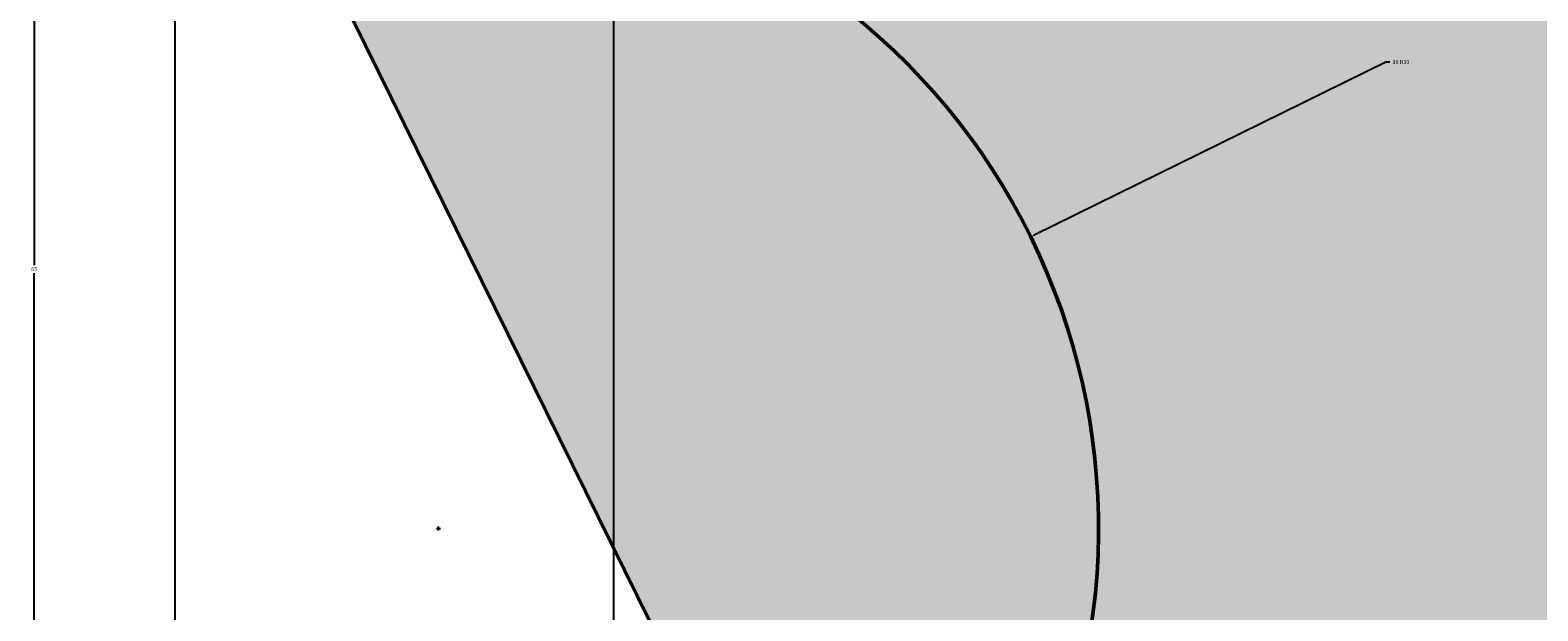
# Model space of a CAD drawing. Units: inches. Extents: x -31 to 87, y -18 to 100.
# Tile 2 of 7: x -31 to 37, y 25 to 52. Entities that reach past the tile are written whole.
import ezdxf

# ---------------------------------------------------------------- set-up
doc = ezdxf.new("R2010")
doc.units = ezdxf.units.IN
doc.header["$MEASUREMENT"] = 0
for name, color, linetype, lineweight in [('M-DIMS', 2, 'Continuous', 18), ('M-HATC', 7, 'Continuous', 18), ('M-OUTL', 4, 'Continuous', 50)]:
    doc.layers.add(name, color=color, linetype=linetype, lineweight=lineweight)
doc.styles.get("Standard").update_dxf_attribs({"font": 'arial.ttf'})
doc.dimstyles.get("Standard").update_dxf_attribs({"dimtxt": 0.18, "dimasz": 0.18, "dimexe": 0.18, "dimexo": 0.0625, "dimgap": 0.09, "dimtad": 0, "dimtih": 1, "dimtoh": 1, "dimdec": 4, "dimzin": 0, "dimdsep": 46, "dimtxsty": 'Standard', "dimcen": 0.09, "dimadec": 0, "dimazin": 0, "dimtfac": 1, "dimtdec": 4, "dimtofl": 0, "dimtmove": 0, "dimatfit": 3, "dimfxl": 1, "dimtolj": 1, "dimtzin": 0, "dimarcsym": 0})

# ---------------------------------------------------------------- blocks, each defined once
blk = doc.blocks.new('*D1')
at = {"layer": 'Defpoints', "color": 0, "transparency": 16777216}
for p in [(-24.622, 75.027), (80.28, 72.235), (80.28, -17.851)]:
    blk.add_point(p, dxfattribs=at)
at = {"layer": 'M-DIMS', "color": 0, "lineweight": -2, "transparency": 16777216}
for p, q in [((-24.622, 74.965), (-24.622, -18.031)), ((80.28, 72.173), (80.28, -18.031)), ((-24.442, -17.851), (27.443, -17.851)), ((80.1, -17.851), (28.214, -17.851))]:
    blk.add_line(p, q, dxfattribs=at)
at = {"layer": 'M-DIMS', "color": 0, "transparency": 16777216}
for points in [[(-24.442, -17.821), (-24.442, -17.881), (-24.622, -17.851)], [(80.1, -17.821), (80.1, -17.881), (80.28, -17.851)]]:
    blk.add_solid(points, dxfattribs=at)
at = {"layer": 'M-DIMS', "color": 0, "transparency": 16777216, "insert": (27.829, -17.851), "char_height": 0.18, "attachment_point": 5}
blk.add_mtext('\\A1;104.9', dxfattribs=at)
blk = doc.blocks.new('*D2')
at = {"layer": 'Defpoints', "color": 0, "transparency": 16777216}
for p in [(60.278, 93.49), (86.68, 93.49), (28.858, -11.451)]:
    blk.add_point(p, dxfattribs=at)
at = {"layer": 'M-DIMS', "color": 0, "lineweight": -2, "transparency": 16777216}
for p, q in [((60.341, 93.49), (86.86, 93.49)), ((86.68, 93.31), (86.68, 41.201)), ((86.68, -11.271), (86.68, 40.838)), ((28.92, -11.451), (86.86, -11.451))]:
    blk.add_line(p, q, dxfattribs=at)
at = {"layer": 'M-DIMS', "color": 0, "transparency": 16777216}
for points in [[(86.65, 93.31), (86.71, 93.31), (86.68, 93.49)], [(86.65, -11.271), (86.71, -11.271), (86.68, -11.451)]]:
    blk.add_solid(points, dxfattribs=at)
at = {"layer": 'M-DIMS', "color": 0, "transparency": 16777216, "insert": (86.68, 41.019), "char_height": 0.18, "attachment_point": 5}
blk.add_mtext('\\A1;104.94', dxfattribs=at)
blk = doc.blocks.new('*D4')
at = {"layer": 'Defpoints', "color": 0, "transparency": 16777216}
for p in [(-4.681, 73.49), (27.319, 8.49), (27.319, -17.851)]:
    blk.add_point(p, dxfattribs=at)
at = {"layer": 'M-DIMS', "color": 0, "lineweight": -2, "transparency": 16777216}
for p, q in [((-4.681, 73.427), (-4.681, -18.031)), ((27.319, 8.427), (27.319, -18.031)), ((-4.501, -17.851), (11.101, -17.851)), ((27.139, -17.851), (11.537, -17.851))]:
    blk.add_line(p, q, dxfattribs=at)
at = {"layer": 'M-DIMS', "color": 0, "transparency": 16777216}
for points in [[(-4.501, -17.821), (-4.501, -17.881), (-4.681, -17.851)], [(27.139, -17.821), (27.139, -17.881), (27.319, -17.851)]]:
    blk.add_solid(points, dxfattribs=at)
at = {"layer": 'M-DIMS', "color": 0, "transparency": 16777216, "insert": (11.319, -17.851), "char_height": 0.18, "attachment_point": 5}
blk.add_mtext('\\A1;32', dxfattribs=at)
blk = doc.blocks.new('*D5')
at = {"layer": 'Defpoints', "color": 0, "transparency": 16777216}
for p in [(-31.022, 73.49), (-4.681, 73.49), (27.319, 8.49)]:
    blk.add_point(p, dxfattribs=at)
at = {"layer": 'M-DIMS', "color": 0, "lineweight": -2, "transparency": 16777216}
for p, q in [((-4.744, 73.49), (-31.202, 73.49)), ((-31.022, 73.31), (-31.022, 41.172)), ((-31.022, 8.67), (-31.022, 40.808)), ((27.256, 8.49), (-31.202, 8.49))]:
    blk.add_line(p, q, dxfattribs=at)
at = {"layer": 'M-DIMS', "color": 0, "transparency": 16777216}
for points in [[(-31.052, 73.31), (-30.992, 73.31), (-31.022, 73.49)], [(-31.052, 8.67), (-30.992, 8.67), (-31.022, 8.49)]]:
    blk.add_solid(points, dxfattribs=at)
at = {"layer": 'M-DIMS', "color": 0, "transparency": 16777216, "insert": (-31.022, 40.99), "char_height": 0.18, "attachment_point": 5}
blk.add_mtext('\\A1;65', dxfattribs=at)
blk = doc.blocks.new('*D9')
at = {"layer": 'Defpoints', "color": 0, "transparency": 16777216}
for p in [(14.282, 42.449), (-12.633, 29.198)]:
    blk.add_point(p, dxfattribs=at)
at = {"layer": 'M-DIMS', "color": 0, "lineweight": -2, "transparency": 16777216}
for p, q in [((30.431, 50.399), (14.443, 42.528)), ((30.611, 50.399), (30.431, 50.399)), ((-12.723, 29.198), (-12.543, 29.198)), ((-12.633, 29.108), (-12.633, 29.288))]:
    blk.add_line(p, q, dxfattribs=at)
at = {"layer": 'M-DIMS', "color": 0, "transparency": 16777216}
blk.add_solid([(14.43, 42.555), (14.456, 42.501), (14.282, 42.449)], dxfattribs=at)
at = {"layer": 'M-DIMS', "color": 0, "transparency": 16777216, "insert": (31.109, 50.399), "char_height": 0.18, "attachment_point": 5}
blk.add_mtext('\\A1;3X R30', dxfattribs=at)

msp = doc.modelspace()

# ---------------------------------------------------------------- hatches: boundary and pattern name
at = {"layer": 'M-HATC'}
h = msp.add_hatch(color=256, dxfattribs=at)
h.set_gradient(color1=(205, 32, 39), color2=(247, 242, 129))
h.paths.add_polyline_path([(-2.425, 93.362, 0.593504), (-22.614, 64.635), (8.64, 1.342, 0.746388), (46.874, 4.293), (79.436, 67.614, 0.505151), (60.278, 93.49)])
h.paths.add_polyline_path([(49.486, 83.865, -1.392259), (62.663, 58.674, 0.510547), (40.663, 15.341, -1.641082), (14.002, 15.393, 0.505248), (-7.332, 58.726, -1.377138), (6.152, 83.865, 0.426931)], flags=16)
h.paths.add_polyline_path([(5.319, 73.49, -1), (-14.681, 73.49, -1)], flags=0)
h.paths.add_polyline_path([(70.319, 73.49, -1), (50.319, 73.49, -1)], flags=0)
h.paths.add_polyline_path([(37.319, 8.49, -1), (17.319, 8.49, -1)], flags=0)
h.paths.add_polyline_path([(6.152, 83.865, 1.377138), (-7.332, 58.726, -0.505248), (14.002, 15.393, 1.641082), (40.663, 15.341, -0.510547), (62.663, 58.674, 1.392259), (49.486, 83.865, -0.426931)], flags=0)

# ---------------------------------------------------------------- linework, layer by layer
at = {"layer": 'M-OUTL'}
msp.add_line((8.64, 1.342), (-22.614, 64.635), dxfattribs=at)
msp.add_arc((-12.633, 29.198), 30, 332.60114, 79.82161, dxfattribs=at)

# ---------------------------------------------------------------- dimensions: what is measured, and where the dimension line sits
at = {"layer": 'M-DIMS'}
for base, p1, p2, override, picture, middle in [((86.68, 93.49), (28.858, -11.451), (60.278, 93.49), {"dimdec": 2, "dimlfac": 1, "dimrnd": 0, "dimzin": 0, "dimdsep": 46, "dimlunit": 2}, '*D2', (86.68, 41.019)), ((-31.022, 73.49), (27.319, 8.49), (-4.681, 73.49), {"dimdec": 0, "dimlfac": 1, "dimrnd": 0, "dimzin": 0, "dimdsep": 46, "dimlunit": 2}, '*D5', (-31.022, 40.99))]:
    dim = msp.add_linear_dim(base=base, p1=p1, p2=p2, angle=90, dimstyle='Standard', override=override, dxfattribs=at)
    dim.commit()
    dim.dimension.update_dxf_attribs({"geometry": picture, "text_midpoint": middle})
for base, p1, p2, override, picture, middle in [((80.28, -17.851), (-24.622, 75.027), (80.28, 72.235), {"dimdec": 1, "dimlfac": 1, "dimrnd": 0, "dimzin": 0, "dimdsep": 46, "dimlunit": 2}, '*D1', (27.829, -17.851)), ((27.319, -17.851), (-4.681, 73.49), (27.319, 8.49), {"dimdec": 0, "dimlfac": 1, "dimrnd": 0, "dimzin": 0, "dimdsep": 46, "dimlunit": 2}, '*D4', (11.319, -17.851))]:
    dim = msp.add_linear_dim(base=base, p1=p1, p2=p2, dimstyle='Standard', override=override, dxfattribs=at)
    dim.commit()
    dim.dimension.update_dxf_attribs({"geometry": picture, "text_midpoint": middle})
dim = msp.add_radius_dim(center=(-12.633, 29.198), mpoint=(14.282, 42.449), text='3X <>', dimstyle='Standard', override={"dimdec": 0, "dimlfac": 1, "dimrnd": 0, "dimzin": 0, "dimdsep": 46, "dimlunit": 2}, dxfattribs=at)
dim.commit()
dim.dimension.update_dxf_attribs({"geometry": '*D9', "text_midpoint": (31.109, 50.399), "dimtype": 164})

doc.saveas('drawing.dxf')
